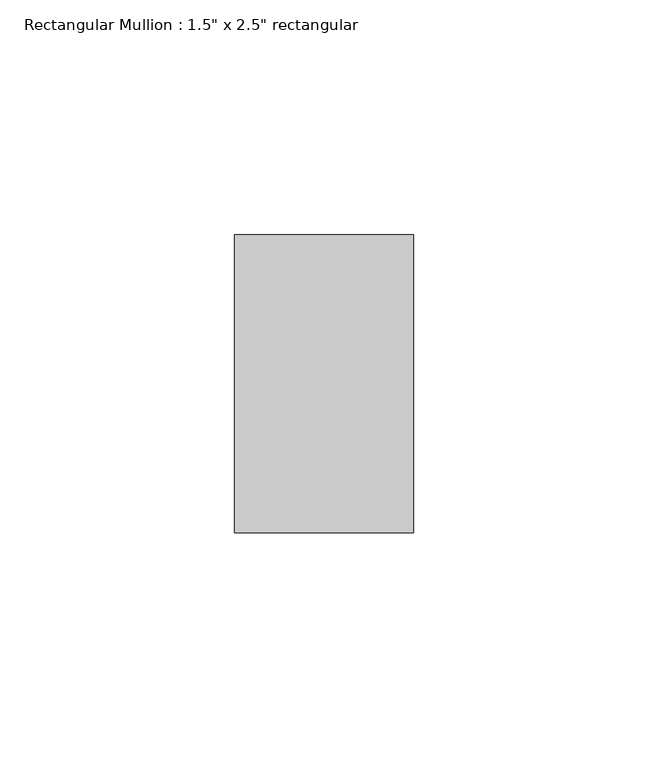
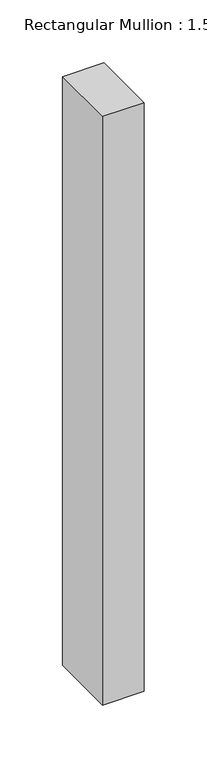
"""IFC4 building model written with IfcOpenShell, lengths in millimetres: member geometry."""

from ifc_helpers import new_model, si_unit, frame, origin, place, context, project, spatial, polyline, outline, extrude, source, transform, mapped, element, save


def member_a67f877f(model_context):
    return source(origin(), model_context, "Body", "SweptSolid", [
        extrude(outline(polyline([(0.0, 31.75), (0.0, -31.75), (-38.1, -31.75), (-38.1, 31.75), (0.0, 31.75)])), frame((0.0, 0.0, -571.5), z_axis=(0.0, 0.0, 1.0), x_axis=(1.0, 0.0, 0.0)), (0.0, 0.0, 1.0), 571.5),
    ])


if __name__ == "__main__":
    model = new_model("IFC4")
    model_context = context("Model", 3, world=origin())
    ifc_project = project(units=[si_unit("LENGTHUNIT", "METRE", prefix="MILLI")], contexts=[model_context])
    site = spatial("IfcSite", under=ifc_project)
    building = spatial("IfcBuilding", under=site)
    placement = place(None, origin())
    member_shape = member_a67f877f(model_context)
    element("IfcMember", 1, ObjectType="Rectangular Mullion : 1.5\" x 2.5\" rectangular", at=placement, inside=building, context=model_context, shape_type="MappedRepresentation", body=[
        mapped(member_shape, transform((0.0, 0.0, 0.0), x_axis=(1.0, 0.0, 0.0), y_axis=(0.0, 1.0, 0.0), z_axis=(0.0, 0.0, 1.0))),
    ])
    save(model, "model.ifc")

# Revit data of these elements
# Type "Rectangular Mullion : 1.5\" x 2.5\" rectangular"
#   built-in parameter 1007304 = 0.208333 (stored number, unit not read)
#   built-in parameter 1007301 = 0.0625 (stored number, unit not read)
#   built-in parameter 1007300 = 0.0625 (stored number, unit not read)
# Element 1 (IfcMember, "Rectangular Mullion : 1.5\" x 2.5\" rectangular")
#   Materials on its faces: "Aluminum"
# Materials
#   "Aluminum": class "Metal", colour RGB 247 247 247, transparency 0, Description = "Aluminum 6061", Cost = 0
